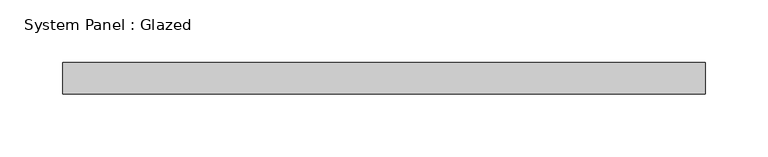
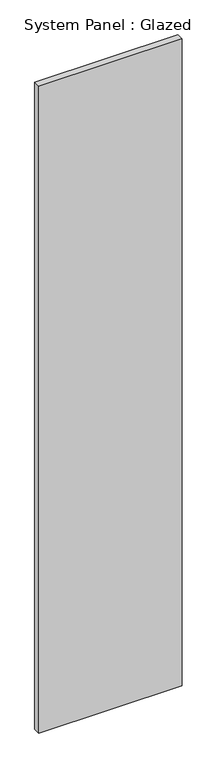
"""IFC4 building model written with IfcOpenShell, lengths in millimetres: plate geometry, System Panel : Glazed."""

from ifc_helpers import new_model, si_unit, origin, origin_with_axes, place, context, project, spatial, polyline, outline, extrude, source, transform, mapped, element, save


def system_panel_glazed_3ac39dea(model_context):
    return source(origin(), model_context, "Body", "SweptSolid", [
        extrude(outline(polyline([(257.175, 19.05), (-257.175, 19.05), (-257.175, 44.45), (257.175, 44.45), (257.175, 19.05)])), origin_with_axes(), (0.0, 0.0, 1.0), 2454.7369027),
    ])


if __name__ == "__main__":
    model = new_model("IFC4")
    model_context = context("Model", 3, world=origin())
    ifc_project = project(units=[si_unit("LENGTHUNIT", "METRE", prefix="MILLI")], contexts=[model_context])
    site = spatial("IfcSite", under=ifc_project)
    building = spatial("IfcBuilding", under=site)
    placement = place(None, origin())
    system_panel_glazed_shape = system_panel_glazed_3ac39dea(model_context)
    element("IfcPlate", 1, ObjectType="System Panel : Glazed", at=placement, inside=building, context=model_context, shape_type="MappedRepresentation", body=[
        mapped(system_panel_glazed_shape, transform((0.0, 0.0, 0.0), x_axis=(1.0, 0.0, 0.0), y_axis=(0.0, 1.0, 0.0), z_axis=(0.0, 0.0, 1.0))),
    ])
    save(model, "model.ifc")

# Revit data of these elements
# Type "System Panel : Glazed"
#   Construction Type Id = "GSP4R"
#   Analytic Construction = "1/8 in Pilkington single glazing"
#   Visual Light Transmittance = 0.9
#   Solar Heat Gain Coefficient = 0.86
#   Heat Transfer Coefficient (U) = 1.18115 BTU/(h·ft²·°F)
#   Define Thermal Properties by = 1
# Element 1 (IfcPlate, "System Panel : Glazed")
#   Materials on its faces: "Glass"
# Materials
#   "Glass": class "Glass", colour RGB 0 128 192, transparency 0.75, Description = "Soda Lime Glass", Cost = 0
